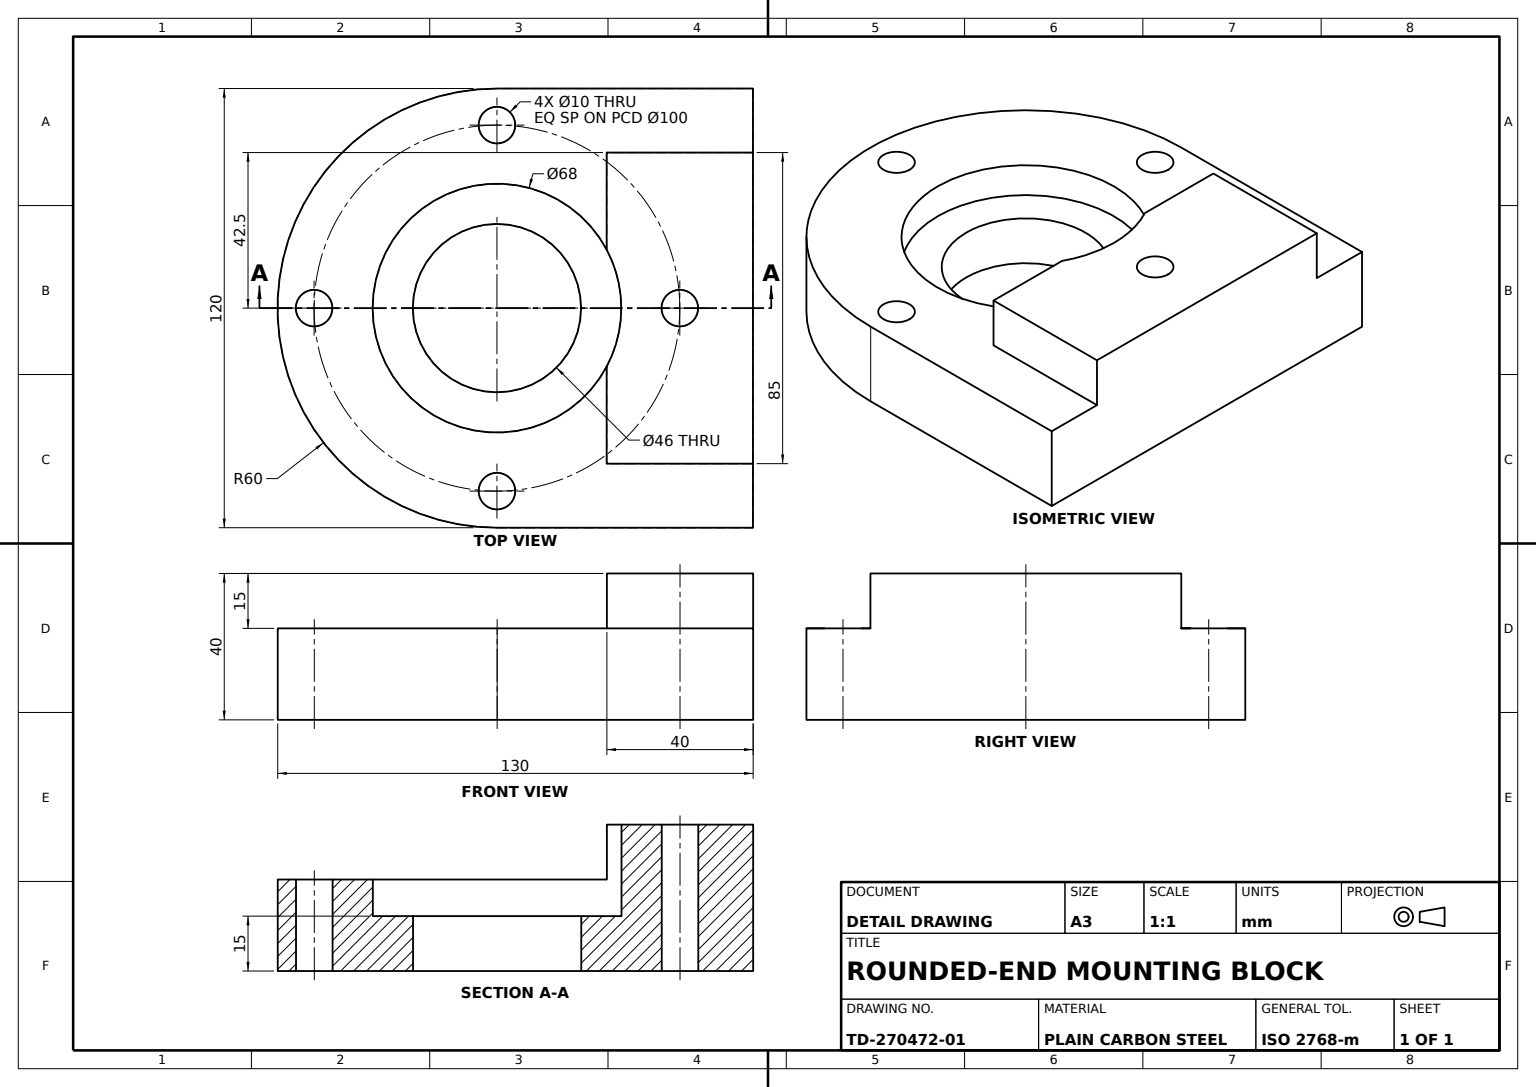
from build123d import *

# Parameters (mm, degrees)
BASE_PLATE_DEPTH          = 25
UPRIGHT_BLOCK_SKETCH_W    = 85
UPRIGHT_BLOCK_SKETCH_H    = 15
UPRIGHT_BLOCK_DEPTH       = 40
MOUNTING_HOLES_SKETCH_R   = 5
MOUNTING_HOLES_CUT_DEPTH  = 40
COUNTERBORE_68_DEPTH      = 40
COUNTERBORE_68_DEPTH_BACK = 10
COUNTERBORE_68_SKETCH_R   = 34
BORE_46_SKETCH_R          = 23
BORE_46_DEPTH             = 15


with BuildPart() as part:
    # Base Plate Sketch → Base Plate (new body)
    with BuildSketch(Plane(origin=(0, 0, 0), x_dir=(1, 0, 0), z_dir=(0, 1, 0))):
        with BuildLine():
            Line((-60, 35), (60, 35))
            Line((60, 35), (60, -35))
            ThreePointArc((60, -35), (0, -95), (-60, -35))
            Line((-60, -35), (-60, 35))
        make_face()
    extrude(amount=BASE_PLATE_DEPTH)

    # Upright Block Sketch → Upright Block (add)
    with BuildSketch(Plane(origin=(0, 0, -35), x_dir=(-1, 0, 0), z_dir=(0, 0, -1))):
        with Locations((0, 32.5)):
            Rectangle(UPRIGHT_BLOCK_SKETCH_W, UPRIGHT_BLOCK_SKETCH_H)
    extrude(amount=-UPRIGHT_BLOCK_DEPTH)

    # Mounting Holes Sketch → Mounting Holes Cut (cut)
    with BuildSketch(Plane(origin=(0, 40, 0), x_dir=(1, 0, 0), z_dir=(0, 1, 0))):
        with Locations(Location((0, 15, 0), (0, 0, 270))):
            Circle(MOUNTING_HOLES_SKETCH_R)
        with Locations(Location((-50, -35, 0), (0, 0, 270))):
            Circle(MOUNTING_HOLES_SKETCH_R)
        with Locations(Location((50, -35, 0), (0, 0, 270))):
            Circle(MOUNTING_HOLES_SKETCH_R)
        with Locations(Location((0, -85, 0), (0, 0, 270))):
            Circle(MOUNTING_HOLES_SKETCH_R)
    extrude(amount=-MOUNTING_HOLES_CUT_DEPTH, mode=Mode.SUBTRACT)

    # Counterbore Ø68 Sketch → Counterbore Ø68 (cut, two sides: drawn at the far end of the back side and taken through both)
    with BuildSketch(Plane(origin=(0, 25, 0), x_dir=(1, 0, 0), z_dir=(0, 1, 0)).offset(-COUNTERBORE_68_DEPTH_BACK)):
        with Locations(Location((0, -35, 0), (0, 0, 61.927513064))):
            Circle(COUNTERBORE_68_SKETCH_R)
    extrude(amount=COUNTERBORE_68_DEPTH + COUNTERBORE_68_DEPTH_BACK, mode=Mode.SUBTRACT)

    # Bore Ø46 Sketch → Bore Ø46 (cut)
    with BuildSketch(Plane(origin=(0, 15, 0), x_dir=(1, 0, 0), z_dir=(0, 1, 0))):
        with Locations(Location((0, -35, 0), (0, 0, 270))):
            Circle(BORE_46_SKETCH_R)
    extrude(amount=-BORE_46_DEPTH, mode=Mode.SUBTRACT)


solid = part.part
